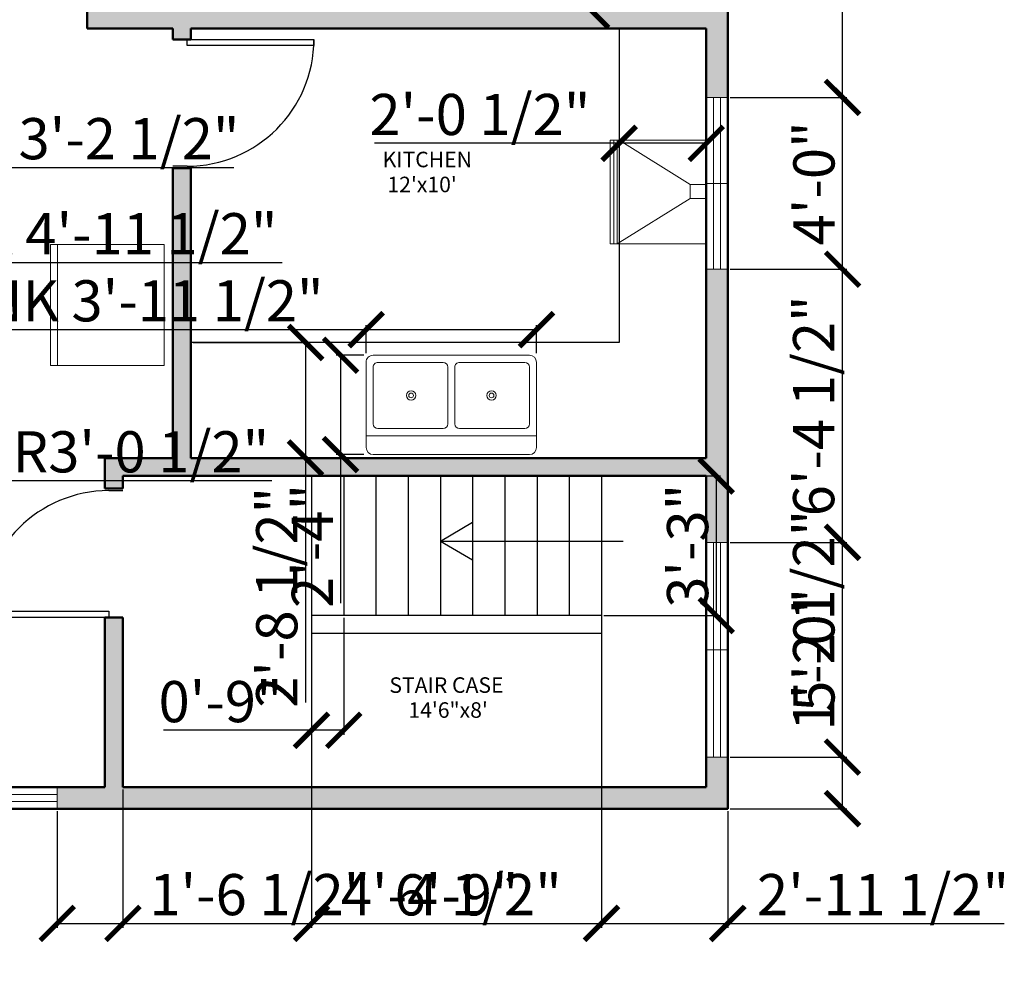
# Model space of a CAD drawing. Units: inches. Extents: x 3147 to 3847, y 1414 to 2207.
# Tile 4 of 7: x 3572 to 3847, y 1452 to 1716. Entities that reach past the tile are written whole.
import ezdxf

# ---------------------------------------------------------------- set-up
doc = ezdxf.new("R2010")
doc.units = ezdxf.units.IN
for name, color, linetype, lineweight in [('A-ANNO-DIMS', 2, 'Continuous', 18), ('A-AREA-IDEN', 7, 'Continuous', 18), ('A-DOOR', 3, 'Continuous', 25), ('A-EQPM', 9, 'Continuous', 18), ('A-FLOR-CASE', 32, 'Continuous', 25), ('A-FLOR-FIXT', 9, 'Continuous', 18), ('A-FLOR-STRS', 7, 'Continuous', 25), ('A-GLAZ', 4, 'Continuous', 18), ('A-WALL', 7, 'Continuous', 50)]:
    doc.layers.add(name, color=color, linetype=linetype, lineweight=lineweight)
doc.layers.add('A-WALL-PATT', color=18, linetype='Continuous', lineweight=13, true_color=0x000000)
doc.styles.get("Standard").update_dxf_attribs({"font": 'arial.ttf'})
doc.dimstyles.new('ISO-25', dxfattribs={"dimtxt": 11.5, "dimasz": 9.5, "dimexe": 1.25, "dimexo": 0.625, "dimtad": 1, "dimdec": 0, "dimlunit": 3, "dimtxsty": 'Standard', "dimblk": 'ARCHTICK', "dimcen": 2.5, "dimadec": 0, "dimazin": 0, "dimtfac": 1, "dimtdec": 0, "dimtmove": 0, "dimatfit": 3, "dimfxl": 1, "dimarcsym": 0})

# ---------------------------------------------------------------- blocks, each defined once
blk = doc.blocks.new('*U6')
for p, q in [((0, 0), (0, -100)), ((900, 0), (900, -100))]:
    blk.add_line(p, q)
blk.add_lwpolyline([(0, 0), (0, 900), (43.75, 900), (43.75, 0)], close=True)
blk.add_arc((0, 0), 900, 0, 90)
blk = doc.blocks.new('Sink-double - 36 in top')
for p, q in [((-18, -4), (18, -4)), ((-0.75, -18.5), (-0.75, -6.5)), ((0.75, -6.5), (0.75, -18.5))]:
    blk.add_line(p, q)
for points in [[(-16.5, 0), (16.5, 0)], [(-18, -19.5), (-18, -1.5)], [(18, -1.5), (18, -19.5)], [(-15.5, -5.5), (-1.75, -5.5)], [(1.75, -5.5), (15.5, -5.5)], [(-16.5, -18.5), (-16.5, -6.5)], [(16.5, -6.5), (16.5, -18.5)], [(-1.75, -19.5), (-15.5, -19.5)], [(15.5, -19.5), (1.75, -19.5)], [(16.5, -21), (-16.5, -21)]]:
    blk.add_lwpolyline(points)
for centre, radius in [((-8.5, -12.5), 1), ((-8.5, -12.5), 0.5), ((8.5, -12.5), 1), ((8.5, -12.5), 0.5)]:
    blk.add_circle(centre, radius)
for centre, radius, start, end in [((-16.5, -1.5), 1.5, 90, 180), ((16.5, -1.5), 1.5, 0, 90), ((-15.5, -6.5), 1, 90, 180), ((-1.75, -6.5), 1, 0, 90), ((1.75, -6.5), 1, 90, 180), ((15.5, -6.5), 1, 0, 90), ((-15.5, -18.5), 1, 180, 270), ((-1.75, -18.5), 1, 270, 0), ((1.75, -18.5), 1, 180, 270), ((15.5, -18.5), 1, 270, 0), ((-16.5, -19.5), 1.5, 180, 270), ((16.5, -19.5), 1.5, 270, 0)]:
    blk.add_arc(centre, radius, start, end)
blk = doc.blocks.new('WIN-48IN-DIVIDED')
for p, q in [((0, 6), (0, 0)), ((24, 6), (24, 0)), ((48, 6), (48, 0)), ((48, 4), (0, 4))]:
    blk.add_line(p, q)
blk.add_lwpolyline([(48, 2), (0, 2)])
blk = doc.blocks.new('_ArchTick')
at = {"color": 0, "linetype": 'ByBlock', "const_width": 0.15}
blk.add_lwpolyline([(-0.5, -0.5), (0.5, 0.5)], dxfattribs=at)
blk = doc.blocks.new('*D41')
at = {"layer": 'A-ANNO-DIMS', "color": 0, "lineweight": -2, "transparency": 16777216}
for p, q in [((3460.68, 1639.4), (3460.68, 1648.92)), ((3520.02, 1639.4), (3520.02, 1648.92)), ((3460.68, 1647.67), (3520.02, 1647.67)), ((3520.02, 1647.67), (3645.23, 1647.67))]:
    blk.add_line(p, q, dxfattribs=at)
at = {"layer": 'Defpoints', "color": 0, "transparency": 16777216}
for p in [(3520.02, 1647.67), (3460.68, 1638.77), (3520.02, 1638.77)]:
    blk.add_point(p, dxfattribs=at)
at = {"layer": 'A-ANNO-DIMS', "color": 0, "lineweight": -2, "transparency": 16777216, "xscale": 9.5, "yscale": 9.5, "zscale": 9.5, "rotation": 180}
blk.add_blockref('_ArchTick', (3460.68, 1647.67), dxfattribs=at)
at = {"layer": 'A-ANNO-DIMS', "color": 0, "lineweight": -2, "transparency": 16777216, "xscale": 9.5, "yscale": 9.5, "zscale": 9.5}
blk.add_blockref('_ArchTick', (3520.02, 1647.67), dxfattribs=at)
at = {"layer": 'A-ANNO-DIMS', "color": 0, "transparency": 16777216, "insert": (3587.38, 1654.25), "char_height": 11.5, "attachment_point": 5}
blk.add_mtext('SOFA 4\'-11 1/2"', dxfattribs=at)
blk = doc.blocks.new('*D45')
at = {"layer": 'A-ANNO-DIMS', "color": 0, "lineweight": -2, "transparency": 16777216}
for p, q in [((3668.72, 1628.92), (3479.75, 1628.92)), ((3668.72, 1622.4), (3668.72, 1630.17)), ((3716.33, 1628.92), (3668.72, 1628.92)), ((3716.33, 1622.4), (3716.33, 1630.17))]:
    blk.add_line(p, q, dxfattribs=at)
at = {"layer": 'Defpoints', "color": 0, "transparency": 16777216}
for p in [(3668.72, 1628.92), (3668.72, 1621.78), (3716.33, 1621.78)]:
    blk.add_point(p, dxfattribs=at)
at = {"layer": 'A-ANNO-DIMS', "color": 0, "lineweight": -2, "transparency": 16777216, "xscale": 9.5, "yscale": 9.5, "zscale": 9.5, "rotation": 180}
blk.add_blockref('_ArchTick', (3668.72, 1628.92), dxfattribs=at)
at = {"layer": 'A-ANNO-DIMS', "color": 0, "lineweight": -2, "transparency": 16777216, "xscale": 9.5, "yscale": 9.5, "zscale": 9.5}
blk.add_blockref('_ArchTick', (3716.33, 1628.92), dxfattribs=at)
at = {"layer": 'A-ANNO-DIMS', "color": 0, "transparency": 16777216, "insert": (3569.49, 1635.5), "char_height": 11.5, "attachment_point": 5}
blk.add_mtext('DOUBLE SINK 3\'-11 1/2"', dxfattribs=at)
blk = doc.blocks.new('*D46')
at = {"layer": 'A-ANNO-DIMS', "color": 0, "lineweight": -2, "transparency": 16777216}
for p, q in [((3668.1, 1621.78), (3660.33, 1621.78)), ((3661.58, 1621.78), (3661.58, 1594.01)), ((3668.1, 1594.01), (3660.33, 1594.01)), ((3661.58, 1594.01), (3661.58, 1552.49))]:
    blk.add_line(p, q, dxfattribs=at)
at = {"layer": 'Defpoints', "color": 0, "transparency": 16777216}
for p in [(3668.72, 1621.78), (3661.58, 1594.01), (3668.72, 1594.01)]:
    blk.add_point(p, dxfattribs=at)
at = {"layer": 'A-ANNO-DIMS', "color": 0, "lineweight": -2, "transparency": 16777216, "xscale": 9.5, "yscale": 9.5, "zscale": 9.5}
for p, rotation in [((3661.58, 1621.78), 90), ((3661.58, 1594.01), 270)]:
    blk.add_blockref('_ArchTick', p, dxfattribs=dict(at, rotation=rotation))
at = {"layer": 'A-ANNO-DIMS', "color": 0, "transparency": 16777216, "insert": (3655.18, 1568.5), "char_height": 11.5, "attachment_point": 5, "rotation": 90}
blk.add_mtext('2\'-4"', dxfattribs=at)
blk = doc.blocks.new('*D50')
at = {"layer": 'A-ANNO-DIMS', "color": 0, "lineweight": -2, "transparency": 16777216}
for p, q in [((3525.21, 1683.16), (3525.21, 1672.98)), ((3563.68, 1683.16), (3563.68, 1672.98)), ((3525.21, 1674.23), (3563.68, 1674.23)), ((3563.68, 1674.23), (3631.79, 1674.23))]:
    blk.add_line(p, q, dxfattribs=at)
at = {"layer": 'Defpoints', "color": 0, "transparency": 16777216}
for p in [(3525.21, 1683.78), (3563.68, 1683.78), (3563.68, 1674.23)]:
    blk.add_point(p, dxfattribs=at)
at = {"layer": 'A-ANNO-DIMS', "color": 0, "lineweight": -2, "transparency": 16777216, "xscale": 9.5, "yscale": 9.5, "zscale": 9.5, "rotation": 180}
blk.add_blockref('_ArchTick', (3525.21, 1674.23), dxfattribs=at)
at = {"layer": 'A-ANNO-DIMS', "color": 0, "lineweight": -2, "transparency": 16777216, "xscale": 9.5, "yscale": 9.5, "zscale": 9.5}
blk.add_blockref('_ArchTick', (3563.68, 1674.23), dxfattribs=at)
at = {"layer": 'A-ANNO-DIMS', "color": 0, "transparency": 16777216, "insert": (3602.48, 1680.81), "char_height": 11.5, "attachment_point": 5}
blk.add_mtext('3\'-2 1/2"', dxfattribs=at)
blk = doc.blocks.new('*D52')
at = {"layer": 'A-ANNO-DIMS', "color": 0, "lineweight": -2, "transparency": 16777216}
for p, q in [((3801.81, 1509.48), (3801.81, 1576.51)), ((3770.39, 1509.48), (3803.06, 1509.48)), ((3801.81, 1495.05), (3801.81, 1509.48)), ((3770.39, 1495.05), (3803.06, 1495.05))]:
    blk.add_line(p, q, dxfattribs=at)
at = {"layer": 'Defpoints', "color": 0, "transparency": 16777216}
for p in [(3769.76, 1509.48), (3801.81, 1509.48), (3769.76, 1495.05)]:
    blk.add_point(p, dxfattribs=at)
at = {"layer": 'A-ANNO-DIMS', "color": 0, "lineweight": -2, "transparency": 16777216, "xscale": 9.5, "yscale": 9.5, "zscale": 9.5}
for p, rotation in [((3801.81, 1509.48), 90), ((3801.81, 1495.05), 270)]:
    blk.add_blockref('_ArchTick', p, dxfattribs=dict(at, rotation=rotation))
at = {"layer": 'A-ANNO-DIMS', "color": 0, "transparency": 16777216, "insert": (3795.24, 1547.75), "char_height": 11.5, "attachment_point": 5, "rotation": 90}
blk.add_mtext('1\'-2 1/2"', dxfattribs=at)
blk = doc.blocks.new('*D53')
at = {"layer": 'A-ANNO-DIMS', "color": 0, "lineweight": -2, "transparency": 16777216}
for p, q in [((3770.39, 1569.48), (3803.06, 1569.48)), ((3801.81, 1509.48), (3801.81, 1569.48)), ((3770.39, 1509.48), (3803.06, 1509.48))]:
    blk.add_line(p, q, dxfattribs=at)
at = {"layer": 'Defpoints', "color": 0, "transparency": 16777216}
for p in [(3769.76, 1569.48), (3801.81, 1569.48), (3769.76, 1509.48)]:
    blk.add_point(p, dxfattribs=at)
at = {"layer": 'A-ANNO-DIMS', "color": 0, "lineweight": -2, "transparency": 16777216, "xscale": 9.5, "yscale": 9.5, "zscale": 9.5}
for p, rotation in [((3801.81, 1569.48), 90), ((3801.81, 1509.48), 270)]:
    blk.add_blockref('_ArchTick', p, dxfattribs=dict(at, rotation=rotation))
at = {"layer": 'A-ANNO-DIMS', "color": 0, "transparency": 16777216, "insert": (3795.32, 1539.48), "char_height": 11.5, "attachment_point": 5, "rotation": 90}
blk.add_mtext('5\'-0"', dxfattribs=at)
blk = doc.blocks.new('*D54')
at = {"layer": 'A-ANNO-DIMS', "color": 0, "lineweight": -2, "transparency": 16777216}
for p, q in [((3770.39, 1645.82), (3803.06, 1645.82)), ((3801.81, 1569.48), (3801.81, 1645.82)), ((3770.39, 1569.48), (3803.06, 1569.48))]:
    blk.add_line(p, q, dxfattribs=at)
at = {"layer": 'Defpoints', "color": 0, "transparency": 16777216}
for p in [(3769.76, 1645.82), (3801.81, 1645.82), (3769.76, 1569.48)]:
    blk.add_point(p, dxfattribs=at)
at = {"layer": 'A-ANNO-DIMS', "color": 0, "lineweight": -2, "transparency": 16777216, "xscale": 9.5, "yscale": 9.5, "zscale": 9.5}
for p, rotation in [((3801.81, 1645.82), 90), ((3801.81, 1569.48), 270)]:
    blk.add_blockref('_ArchTick', p, dxfattribs=dict(at, rotation=rotation))
at = {"layer": 'A-ANNO-DIMS', "color": 0, "transparency": 16777216, "insert": (3795.24, 1607.65), "char_height": 11.5, "attachment_point": 5, "rotation": 90}
blk.add_mtext('6\'-4 1/2"', dxfattribs=at)
blk = doc.blocks.new('*D55')
at = {"layer": 'A-ANNO-DIMS', "color": 0, "lineweight": -2, "transparency": 16777216}
for p, q in [((3770.39, 1693.82), (3803.06, 1693.82)), ((3801.81, 1645.82), (3801.81, 1693.82)), ((3770.39, 1645.82), (3803.06, 1645.82))]:
    blk.add_line(p, q, dxfattribs=at)
at = {"layer": 'Defpoints', "color": 0, "transparency": 16777216}
for p in [(3769.76, 1693.82), (3801.81, 1693.82), (3769.76, 1645.82)]:
    blk.add_point(p, dxfattribs=at)
at = {"layer": 'A-ANNO-DIMS', "color": 0, "lineweight": -2, "transparency": 16777216, "xscale": 9.5, "yscale": 9.5, "zscale": 9.5}
for p, rotation in [((3801.81, 1693.82), 90), ((3801.81, 1645.82), 270)]:
    blk.add_blockref('_ArchTick', p, dxfattribs=dict(at, rotation=rotation))
at = {"layer": 'A-ANNO-DIMS', "color": 0, "transparency": 16777216, "insert": (3795.32, 1669.82), "char_height": 11.5, "attachment_point": 5, "rotation": 90}
blk.add_mtext('4\'-0"', dxfattribs=at)
blk = doc.blocks.new('*D56')
at = {"layer": 'A-ANNO-DIMS', "color": 0, "lineweight": -2, "transparency": 16777216}
for p, q in [((3801.81, 1731.24), (3801.81, 1799.35)), ((3770.39, 1731.24), (3803.06, 1731.24)), ((3801.81, 1693.82), (3801.81, 1731.24)), ((3770.39, 1693.82), (3803.06, 1693.82))]:
    blk.add_line(p, q, dxfattribs=at)
at = {"layer": 'Defpoints', "color": 0, "transparency": 16777216}
for p in [(3769.76, 1731.24), (3801.81, 1731.24), (3769.76, 1693.82)]:
    blk.add_point(p, dxfattribs=at)
at = {"layer": 'A-ANNO-DIMS', "color": 0, "lineweight": -2, "transparency": 16777216, "xscale": 9.5, "yscale": 9.5, "zscale": 9.5}
for p, rotation in [((3801.81, 1731.24), 90), ((3801.81, 1693.82), 270)]:
    blk.add_blockref('_ArchTick', p, dxfattribs=dict(at, rotation=rotation))
at = {"layer": 'A-ANNO-DIMS', "color": 0, "transparency": 16777216, "insert": (3795.24, 1770.05), "char_height": 11.5, "attachment_point": 5, "rotation": 90}
blk.add_mtext('3\'-1 1/2"', dxfattribs=at)
blk = doc.blocks.new('*D71')
at = {"layer": 'A-ANNO-DIMS', "color": 0, "lineweight": -2, "transparency": 16777216}
for p, q in [((3600.76, 1500.42), (3600.76, 1461.75)), ((3582.41, 1494.42), (3582.41, 1461.75)), ((3582.41, 1463), (3600.76, 1463)), ((3600.76, 1463), (3667.8, 1463))]:
    blk.add_line(p, q, dxfattribs=at)
at = {"layer": 'Defpoints', "color": 0, "transparency": 16777216}
for p in [(3600.76, 1501.05), (3582.41, 1495.05), (3600.76, 1463)]:
    blk.add_point(p, dxfattribs=at)
at = {"layer": 'A-ANNO-DIMS', "color": 0, "lineweight": -2, "transparency": 16777216, "xscale": 9.5, "yscale": 9.5, "zscale": 9.5, "rotation": 180}
blk.add_blockref('_ArchTick', (3582.41, 1463), dxfattribs=at)
at = {"layer": 'A-ANNO-DIMS', "color": 0, "lineweight": -2, "transparency": 16777216, "xscale": 9.5, "yscale": 9.5, "zscale": 9.5}
blk.add_blockref('_ArchTick', (3600.76, 1463), dxfattribs=at)
at = {"layer": 'A-ANNO-DIMS', "color": 0, "transparency": 16777216, "insert": (3639.03, 1469.57), "char_height": 11.5, "attachment_point": 5}
blk.add_mtext('1\'-6 1/2"', dxfattribs=at)
blk = doc.blocks.new('*D72')
at = {"layer": 'A-ANNO-DIMS', "color": 0, "lineweight": -2, "transparency": 16777216}
for p, q in [((3653.47, 1548.42), (3653.47, 1461.75)), ((3600.76, 1500.42), (3600.76, 1461.75)), ((3600.76, 1463), (3653.47, 1463)), ((3653.47, 1463), (3722.05, 1463))]:
    blk.add_line(p, q, dxfattribs=at)
at = {"layer": 'Defpoints', "color": 0, "transparency": 16777216}
for p in [(3653.47, 1549.05), (3600.76, 1501.05), (3653.47, 1463)]:
    blk.add_point(p, dxfattribs=at)
at = {"layer": 'A-ANNO-DIMS', "color": 0, "lineweight": -2, "transparency": 16777216, "xscale": 9.5, "yscale": 9.5, "zscale": 9.5, "rotation": 180}
blk.add_blockref('_ArchTick', (3600.76, 1463), dxfattribs=at)
at = {"layer": 'A-ANNO-DIMS', "color": 0, "lineweight": -2, "transparency": 16777216, "xscale": 9.5, "yscale": 9.5, "zscale": 9.5}
blk.add_blockref('_ArchTick', (3653.47, 1463), dxfattribs=at)
at = {"layer": 'A-ANNO-DIMS', "color": 0, "transparency": 16777216, "insert": (3692.51, 1469.57), "char_height": 11.5, "attachment_point": 5}
blk.add_mtext('4\'-4 1/2"', dxfattribs=at)
blk = doc.blocks.new('*D73')
at = {"layer": 'A-ANNO-DIMS', "color": 0, "lineweight": -2, "transparency": 16777216}
for p, q in [((3653.47, 1548.42), (3653.47, 1461.75)), ((3734.47, 1548.42), (3734.47, 1461.75)), ((3653.47, 1463), (3734.47, 1463))]:
    blk.add_line(p, q, dxfattribs=at)
at = {"layer": 'Defpoints', "color": 0, "transparency": 16777216}
for p in [(3653.47, 1549.05), (3734.47, 1549.05), (3734.47, 1463)]:
    blk.add_point(p, dxfattribs=at)
at = {"layer": 'A-ANNO-DIMS', "color": 0, "lineweight": -2, "transparency": 16777216, "xscale": 9.5, "yscale": 9.5, "zscale": 9.5, "rotation": 180}
blk.add_blockref('_ArchTick', (3653.47, 1463), dxfattribs=at)
at = {"layer": 'A-ANNO-DIMS', "color": 0, "lineweight": -2, "transparency": 16777216, "xscale": 9.5, "yscale": 9.5, "zscale": 9.5}
blk.add_blockref('_ArchTick', (3734.47, 1463), dxfattribs=at)
at = {"layer": 'A-ANNO-DIMS', "color": 0, "transparency": 16777216, "insert": (3693.97, 1469.5), "char_height": 11.5, "attachment_point": 5}
blk.add_mtext('6\'-9"', dxfattribs=at)
blk = doc.blocks.new('*D74')
at = {"layer": 'A-ANNO-DIMS', "color": 0, "lineweight": -2, "transparency": 16777216}
for p, q in [((3734.47, 1548.42), (3734.47, 1461.75)), ((3769.76, 1494.42), (3769.76, 1461.75)), ((3734.47, 1463), (3769.76, 1463)), ((3769.76, 1463), (3847.01, 1463))]:
    blk.add_line(p, q, dxfattribs=at)
at = {"layer": 'Defpoints', "color": 0, "transparency": 16777216}
for p in [(3734.47, 1549.05), (3769.76, 1495.05), (3769.76, 1463)]:
    blk.add_point(p, dxfattribs=at)
at = {"layer": 'A-ANNO-DIMS', "color": 0, "lineweight": -2, "transparency": 16777216, "xscale": 9.5, "yscale": 9.5, "zscale": 9.5, "rotation": 180}
blk.add_blockref('_ArchTick', (3734.47, 1463), dxfattribs=at)
at = {"layer": 'A-ANNO-DIMS', "color": 0, "lineweight": -2, "transparency": 16777216, "xscale": 9.5, "yscale": 9.5, "zscale": 9.5}
blk.add_blockref('_ArchTick', (3769.76, 1463), dxfattribs=at)
at = {"layer": 'A-ANNO-DIMS', "color": 0, "transparency": 16777216, "insert": (3813.14, 1469.57), "char_height": 11.5, "attachment_point": 5}
blk.add_mtext('2\'-11 1/2"', dxfattribs=at)
blk = doc.blocks.new('*D88')
at = {"layer": 'A-ANNO-DIMS', "color": 0, "lineweight": -2, "transparency": 16777216}
for p, q in [((3763.14, 1849.05), (3730.46, 1849.05)), ((3731.71, 1718.05), (3731.71, 1849.05)), ((3763.14, 1718.05), (3730.46, 1718.05))]:
    blk.add_line(p, q, dxfattribs=at)
at = {"layer": 'Defpoints', "color": 0, "transparency": 16777216}
for p in [(3731.71, 1849.05), (3763.76, 1849.05), (3763.76, 1718.05)]:
    blk.add_point(p, dxfattribs=at)
at = {"layer": 'A-ANNO-DIMS', "color": 0, "lineweight": -2, "transparency": 16777216, "xscale": 9.5, "yscale": 9.5, "zscale": 9.5}
for p, rotation in [((3731.71, 1849.05), 90), ((3731.71, 1718.05), 270)]:
    blk.add_blockref('_ArchTick', p, dxfattribs=dict(at, rotation=rotation))
at = {"layer": 'A-ANNO-DIMS', "color": 0, "transparency": 16777216, "insert": (3725.22, 1783.55), "char_height": 11.5, "attachment_point": 5, "rotation": 90}
blk.add_mtext('10\'-11"', dxfattribs=at)
blk = doc.blocks.new('*D90')
at = {"layer": 'A-ANNO-DIMS', "color": 0, "lineweight": -2, "transparency": 16777216}
for p, q in [((3735.1, 1588.05), (3767.77, 1588.05)), ((3766.52, 1588.05), (3766.52, 1549.05)), ((3735.1, 1549.05), (3767.77, 1549.05))]:
    blk.add_line(p, q, dxfattribs=at)
at = {"layer": 'Defpoints', "color": 0, "transparency": 16777216}
for p in [(3734.47, 1588.05), (3734.47, 1549.05), (3766.52, 1549.05)]:
    blk.add_point(p, dxfattribs=at)
at = {"layer": 'A-ANNO-DIMS', "color": 0, "lineweight": -2, "transparency": 16777216, "xscale": 9.5, "yscale": 9.5, "zscale": 9.5}
for p, rotation in [((3766.52, 1588.05), 90), ((3766.52, 1549.05), 270)]:
    blk.add_blockref('_ArchTick', p, dxfattribs=dict(at, rotation=rotation))
at = {"layer": 'A-ANNO-DIMS', "color": 0, "transparency": 16777216, "insert": (3760.02, 1568.55), "char_height": 11.5, "attachment_point": 5, "rotation": 90}
blk.add_mtext('3\'-3"', dxfattribs=at)
blk = doc.blocks.new('*D91')
at = {"layer": 'A-ANNO-DIMS', "color": 0, "lineweight": -2, "transparency": 16777216}
for p, q in [((3653.47, 1548.42), (3653.47, 1515.75)), ((3662.47, 1548.42), (3662.47, 1515.75)), ((3653.47, 1517), (3612.15, 1517)), ((3662.47, 1517), (3653.47, 1517))]:
    blk.add_line(p, q, dxfattribs=at)
at = {"layer": 'Defpoints', "color": 0, "transparency": 16777216}
for p in [(3653.47, 1549.05), (3662.47, 1549.05), (3653.47, 1517)]:
    blk.add_point(p, dxfattribs=at)
at = {"layer": 'A-ANNO-DIMS', "color": 0, "lineweight": -2, "transparency": 16777216, "xscale": 9.5, "yscale": 9.5, "zscale": 9.5, "rotation": 180}
blk.add_blockref('_ArchTick', (3653.47, 1517), dxfattribs=at)
at = {"layer": 'A-ANNO-DIMS', "color": 0, "lineweight": -2, "transparency": 16777216, "xscale": 9.5, "yscale": 9.5, "zscale": 9.5}
blk.add_blockref('_ArchTick', (3662.47, 1517), dxfattribs=at)
at = {"layer": 'A-ANNO-DIMS', "color": 0, "transparency": 16777216, "insert": (3628.06, 1523.5), "char_height": 11.5, "attachment_point": 5}
blk.add_mtext('0\'-9"', dxfattribs=at)
blk = doc.blocks.new('*D92')
at = {"layer": 'A-ANNO-DIMS', "color": 0, "lineweight": -2, "transparency": 16777216}
for p, q in [((3620.39, 1625.36), (3653.06, 1625.36)), ((3651.81, 1625.36), (3651.81, 1593.05)), ((3620.39, 1593.05), (3653.06, 1593.05)), ((3651.81, 1593.05), (3651.81, 1524.74))]:
    blk.add_line(p, q, dxfattribs=at)
at = {"layer": 'Defpoints', "color": 0, "transparency": 16777216}
for p in [(3619.76, 1625.36), (3619.76, 1593.05), (3651.81, 1593.05)]:
    blk.add_point(p, dxfattribs=at)
at = {"layer": 'A-ANNO-DIMS', "color": 0, "lineweight": -2, "transparency": 16777216, "xscale": 9.5, "yscale": 9.5, "zscale": 9.5}
for p, rotation in [((3651.81, 1625.36), 90), ((3651.81, 1593.05), 270)]:
    blk.add_blockref('_ArchTick', p, dxfattribs=dict(at, rotation=rotation))
at = {"layer": 'A-ANNO-DIMS', "color": 0, "transparency": 16777216, "insert": (3645.24, 1554.14), "char_height": 11.5, "attachment_point": 5, "rotation": 90}
blk.add_mtext('2\'-8 1/2"', dxfattribs=at)
blk = doc.blocks.new('*D93')
at = {"layer": 'A-ANNO-DIMS', "color": 0, "lineweight": -2, "transparency": 16777216}
for p, q in [((3739.42, 1712.42), (3739.42, 1679.75)), ((3763.76, 1712.42), (3763.76, 1679.75)), ((3739.42, 1681), (3671.1, 1681)), ((3763.76, 1681), (3739.42, 1681))]:
    blk.add_line(p, q, dxfattribs=at)
at = {"layer": 'Defpoints', "color": 0, "transparency": 16777216}
for p in [(3739.42, 1713.05), (3763.76, 1713.05), (3739.42, 1681)]:
    blk.add_point(p, dxfattribs=at)
at = {"layer": 'A-ANNO-DIMS', "color": 0, "lineweight": -2, "transparency": 16777216, "xscale": 9.5, "yscale": 9.5, "zscale": 9.5, "rotation": 180}
blk.add_blockref('_ArchTick', (3739.42, 1681), dxfattribs=at)
at = {"layer": 'A-ANNO-DIMS', "color": 0, "lineweight": -2, "transparency": 16777216, "xscale": 9.5, "yscale": 9.5, "zscale": 9.5}
blk.add_blockref('_ArchTick', (3763.76, 1681), dxfattribs=at)
at = {"layer": 'A-ANNO-DIMS', "color": 0, "transparency": 16777216, "insert": (3700.51, 1687.57), "char_height": 11.5, "attachment_point": 5}
blk.add_mtext('2\'-0 1/2"', dxfattribs=at)
blk = doc.blocks.new('*D98')
at = {"layer": 'A-ANNO-DIMS', "color": 0, "lineweight": -2, "transparency": 16777216}
for p in [(3492.69, 1586.73), (3642.35, 1586.73)]:
    blk.add_line(p, (3529.03, 1586.73), dxfattribs=at)
at = {"layer": 'Defpoints', "color": 0, "transparency": 16777216}
for p in [(3492.69, 1586.73), (3529.03, 1586.73)]:
    blk.add_point(p, dxfattribs=at)
at = {"layer": 'A-ANNO-DIMS', "color": 0, "lineweight": -2, "transparency": 16777216, "xscale": 9.5, "yscale": 9.5, "zscale": 9.5, "rotation": 180.0000425795118}
blk.add_blockref('_ArchTick', (3529.03, 1586.73), dxfattribs=at)
at = {"layer": 'A-ANNO-DIMS', "color": 0, "transparency": 16777216, "insert": (3595.19, 1593.3), "char_height": 11.5, "attachment_point": 5, "rotation": 0}
blk.add_mtext('3X R3\'-0 1/2"', dxfattribs=at)

msp = doc.modelspace()

# ---------------------------------------------------------------- hatches: boundary and pattern name
at = {"layer": 'A-WALL-PATT'}
h = msp.add_hatch(color=256, dxfattribs=at)
h.dxf.hatch_style = 1
h.paths.add_polyline_path([(3616.76, 2093.05), (3594.02, 2093.05), (3594.02, 2087.05), (3611.76, 2087.05), (3611.76, 1993.05), (3616.76, 1993.05), (3628.76, 1993.05), (3628.76, 1996.99), (3628.76, 1998.05), (3616.76, 1998.05), (3616.76, 2087.05)])
h.paths.add_polyline_path([(3576.44, 2093.05), (3527.03, 2093.05), (3527.03, 2087.05), (3546.76, 2087.05), (3546.76, 1962.05), (3551.76, 1962.05), (3590.76, 1962.05), (3590.76, 1921.05), (3585.76, 1921.05), (3585.76, 1916.05), (3590.76, 1916.05), (3590.76, 1895.05), (3595.76, 1895.05), (3595.76, 1962.05), (3611.76, 1962.05), (3616.76, 1962.05), (3616.76, 1969.05), (3611.76, 1969.05), (3611.76, 1967.05), (3551.76, 1967.05), (3551.76, 2087.05), (3576.44, 2087.05)])
h.paths.add_polyline_path([(3455.03, 2093.05), (3408.76, 2093.05), (3408.76, 2087.05), (3408.76, 2046.06), (3413.76, 2046.06), (3413.76, 2087.05), (3455.03, 2087.05)])
h.paths.add_polyline_path([(3355.76, 2008.05), (3408.76, 2008.05), (3408.76, 2004.83), (3413.76, 2004.83), (3413.76, 2008.05), (3413.76, 2013.05), (3413.76, 2016.06), (3408.76, 2016.06), (3408.76, 2013.05), (3355.76, 2013.05), (3349.76, 2013.05), (3349.76, 1973.71), (3355.76, 1973.71)])
h.paths.add_polyline_path([(3413.76, 1974.83), (3408.76, 1974.83), (3408.76, 1943.05), (3355.76, 1943.05), (3355.76, 1949.71), (3349.76, 1949.71), (3349.76, 1897.34), (3355.76, 1897.34), (3355.76, 1938.05), (3408.76, 1938.05), (3408.76, 1934.63), (3413.76, 1934.63), (3413.76, 1938.05), (3505.76, 1938.05), (3505.76, 1916.05), (3533.76, 1916.05), (3533.76, 1904.63), (3533.76, 1831.83), (3538.76, 1831.83), (3538.76, 1904.63), (3538.76, 1916.05), (3546.76, 1916.05), (3549.76, 1916.05), (3549.76, 1921.05), (3546.76, 1921.05), (3510.76, 1921.05), (3510.76, 1938.05), (3510.76, 1943.05), (3413.76, 1943.05)])
h.paths.add_polyline_path([(3413.76, 1904.63), (3408.76, 1904.63), (3408.76, 1870.05), (3355.76, 1870.05), (3355.76, 1873.34), (3349.76, 1873.34), (3349.76, 1865.05), (3355.76, 1865.05), (3408.76, 1865.05), (3408.76, 1863.11), (3409.83, 1863.11), (3413.76, 1863.11)], flags=17)
h.paths.add_polyline_path([(3538.76, 1795.83), (3533.76, 1795.83), (3533.76, 1794.05), (3413.76, 1794.05), (3413.76, 1833.11), (3408.76, 1833.11), (3408.76, 1794.05), (3355.76, 1794.05), (3349.76, 1794.05), (3349.76, 1776.88), (3355.76, 1776.88), (3355.76, 1789.05), (3413.76, 1789.05), (3475.76, 1789.05), (3475.76, 1731.91), (3480.76, 1731.91), (3480.76, 1789.05), (3538.76, 1789.05)])
h.paths.add_polyline_path([(3432.14, 1733.05), (3413.76, 1733.05), (3355.76, 1733.05), (3355.76, 1740.88), (3349.76, 1740.88), (3349.76, 1720.47), (3355.76, 1720.47), (3355.76, 1729.05), (3413.76, 1729.05), (3432.14, 1729.05)])
h.paths.add_polyline_path([(3480.76, 1695.91), (3476.83, 1695.91), (3475.76, 1695.91), (3475.76, 1693.05), (3413.76, 1693.05), (3355.76, 1693.05), (3355.76, 1696.47), (3349.76, 1696.47), (3349.76, 1671.27), (3355.76, 1671.27), (3355.76, 1688.05), (3413.76, 1688.05), (3415.76, 1688.05), (3415.76, 1673.71), (3420.76, 1673.71), (3420.76, 1688.05), (3480.76, 1688.05)])
h.paths.add_polyline_path([(3420.76, 1643.71), (3415.76, 1643.71), (3415.76, 1642.05), (3413.76, 1642.05), (3355.76, 1642.05), (3355.76, 1647.27), (3349.76, 1647.27), (3349.76, 1598.35), (3355.76, 1598.35), (3355.76, 1637.05), (3401.76, 1637.05), (3401.76, 1634.26), (3406.76, 1634.26), (3406.76, 1637.05), (3413.76, 1637.05), (3420.76, 1637.05)])
h.paths.add_polyline_path([(3406.76, 1604.26), (3401.76, 1604.26), (3401.76, 1572.05), (3355.76, 1572.05), (3355.76, 1574.35), (3349.76, 1574.35), (3349.76, 1553.05), (3349.76, 1495.05), (3371.89, 1495.05), (3371.89, 1501.05), (3355.76, 1501.05), (3355.76, 1559.05), (3355.76, 1567.05), (3406.76, 1567.05), (3406.76, 1572.05)])
h.paths.add_polyline_path([(3534.41, 1501.05), (3419.89, 1501.05), (3419.89, 1495.05), (3534.41, 1495.05)])
h.paths.add_polyline_path([(3769.76, 1509.48), (3763.76, 1509.48), (3763.76, 1501.05), (3600.76, 1501.05), (3600.76, 1548.51), (3595.76, 1548.51), (3595.76, 1501.05), (3582.41, 1501.05), (3582.41, 1495.05), (3769.76, 1495.05)])
h.paths.add_polyline_path([(3769.76, 1645.82), (3763.76, 1645.82), (3763.76, 1593.05), (3664.76, 1593.05), (3619.76, 1593.05), (3619.76, 1674.05), (3614.76, 1674.05), (3614.76, 1593.05), (3595.76, 1593.05), (3595.76, 1584.51), (3600.76, 1584.51), (3600.76, 1588.05), (3619.76, 1588.05), (3664.76, 1588.05), (3763.76, 1588.05), (3763.76, 1569.48), (3769.76, 1569.48)])
h.paths.add_polyline_path([(3769.76, 1731.24), (3763.76, 1731.24), (3763.76, 1718.05), (3664.76, 1718.05), (3595.76, 1718.05), (3595.76, 1723.05), (3590.76, 1723.05), (3590.76, 1713.05), (3595.76, 1713.05), (3614.76, 1713.05), (3614.76, 1710.05), (3619.76, 1710.05), (3619.76, 1713.05), (3664.76, 1713.05), (3763.76, 1713.05), (3763.76, 1693.82), (3769.76, 1693.82)])
h.paths.add_polyline_path([(3769.76, 1872.64), (3763.76, 1872.64), (3763.76, 1854.05), (3664.76, 1854.05), (3595.76, 1854.05), (3595.76, 1859.05), (3590.76, 1859.05), (3590.76, 1759.05), (3595.76, 1759.05), (3595.76, 1849.05), (3664.76, 1849.05), (3763.76, 1849.05), (3763.76, 1815.24), (3769.76, 1815.24)])
h.paths.add_polyline_path([(3769.76, 1998.05), (3763.76, 1998.05), (3763.76, 1968.64), (3769.76, 1968.64)])
h.paths.add_polyline_path([(3763.76, 1998.05), (3664.76, 1998.05), (3664.76, 1993.05), (3763.76, 1993.05)])

# ---------------------------------------------------------------- linework, layer by layer
at = {"layer": 'A-EQPM'}
for p, q in [((3736.9, 1652.92), (3736.9, 1681.84)), ((3736.9, 1681.84), (3738.9, 1681.84)), ((3737.9, 1652.92), (3737.9, 1681.84)), ((3738.9, 1681.84), (3763.76, 1681.84)), ((3738.9, 1652.92), (3738.9, 1681.84)), ((3739.42, 1681.84), (3759.29, 1669.49)), ((3763.76, 1681.84), (3763.76, 1652.92)), ((3759.29, 1665.54), (3738.9, 1652.92)), ((3580.52, 1652.72), (3612.29, 1652.72)), ((3580.52, 1618.87), (3580.52, 1652.72)), ((3582.52, 1618.87), (3582.52, 1652.72)), ((3612.29, 1652.72), (3612.29, 1618.87)), ((3736.9, 1652.92), (3738.9, 1652.92)), ((3763.76, 1652.92), (3738.9, 1652.92)), ((3612.29, 1618.87), (3580.52, 1618.87))]:
    msp.add_line(p, q, dxfattribs=at)
msp.add_lwpolyline([(3759.29, 1669.49), (3763.76, 1669.49), (3763.76, 1665.54), (3759.29, 1665.54)], close=True, dxfattribs=at)
at = {"layer": 'A-FLOR-CASE'}
for p, q in [((3739.42, 1713.05), (3739.42, 1625.36)), ((3739.42, 1625.36), (3619.76, 1625.36))]:
    msp.add_line(p, q, dxfattribs=at)
at = {"layer": 'A-FLOR-STRS'}
for p, q in [((3653.47, 1588.05), (3653.47, 1501.05)), ((3662.47, 1588.05), (3662.47, 1549.05)), ((3671.47, 1588.05), (3671.47, 1549.05)), ((3680.47, 1588.05), (3680.47, 1549.05)), ((3689.47, 1588.05), (3689.47, 1549.05)), ((3698.47, 1588.05), (3698.47, 1549.05)), ((3707.47, 1588.05), (3707.47, 1549.05)), ((3716.47, 1588.05), (3716.47, 1549.05)), ((3725.47, 1588.05), (3725.47, 1549.05)), ((3734.47, 1588.05), (3734.47, 1501.05)), ((3689.47, 1569.85), (3698.47, 1575.11)), ((3689.47, 1569.85), (3698.47, 1564.59)), ((3689.47, 1569.85), (3740.56, 1569.85))]:
    msp.add_line(p, q, dxfattribs=at)
for points in [[(3734.47, 1549.05), (3664.76, 1549.05), (3653.47, 1549.05)], [(3734.47, 1544.05), (3664.76, 1544.05), (3653.47, 1544.05)]]:
    msp.add_lwpolyline(points, dxfattribs=at)
at = {"layer": 'A-GLAZ'}
for p, q in [((3763.76, 1693.82), (3769.76, 1693.82)), ((3765.76, 1693.82), (3765.76, 1645.82)), ((3767.76, 1693.82), (3767.76, 1645.82)), ((3763.76, 1669.82), (3769.76, 1669.82)), ((3763.76, 1645.82), (3769.76, 1645.82)), ((3763.76, 1569.48), (3769.76, 1569.48)), ((3765.76, 1569.48), (3765.76, 1509.48)), ((3767.76, 1569.48), (3767.76, 1553.05)), ((3763.76, 1539.48), (3769.76, 1539.48)), ((3763.76, 1509.48), (3769.76, 1509.48))]:
    msp.add_line(p, q, dxfattribs=at)
msp.add_lwpolyline([(3767.76, 1553.05), (3767.76, 1509.48)], dxfattribs=at)
at = {"layer": 'A-WALL'}
for p, q in [((3769.76, 2093.05), (3769.76, 1553.05)), ((3590.76, 1723.05), (3590.76, 1713.05)), ((3595.76, 1713.05), (3590.76, 1713.05)), ((3614.76, 1713.05), (3614.76, 1710.05)), ((3619.76, 1713.05), (3619.76, 1710.05)), ((3763.76, 1713.05), (3763.76, 1593.05)), ((3614.76, 1674.05), (3614.76, 1593.05)), ((3619.76, 1674.05), (3619.76, 1593.05)), ((3614.76, 1593.05), (3595.76, 1593.05)), ((3595.76, 1593.05), (3595.76, 1584.51)), ((3619.76, 1588.05), (3600.76, 1588.05)), ((3600.76, 1588.05), (3600.76, 1584.51)), ((3763.76, 1588.05), (3763.76, 1501.05)), ((3595.76, 1584.51), (3600.76, 1584.51)), ((3595.76, 1548.51), (3595.76, 1501.05)), ((3595.76, 1548.51), (3600.76, 1548.51)), ((3600.76, 1548.51), (3600.76, 1501.05)), ((3595.76, 1501.05), (3355.76, 1501.05)), ((3763.76, 1501.05), (3600.76, 1501.05))]:
    msp.add_line(p, q, dxfattribs=at)
for points in [[(3614.76, 1713.05), (3595.76, 1713.05)], [(3763.76, 1713.05), (3664.76, 1713.05), (3619.76, 1713.05)], [(3619.76, 1710.05), (3614.76, 1710.05)], [(3619.76, 1674.05), (3614.76, 1674.05)], [(3763.76, 1593.05), (3664.76, 1593.05), (3619.76, 1593.05)], [(3763.76, 1588.05), (3664.76, 1588.05), (3614.76, 1588.05)], [(3769.76, 1553.05), (3769.76, 1495.05), (3349.76, 1495.05), (3349.76, 1553.05)]]:
    msp.add_lwpolyline(points, dxfattribs=at)

# ---------------------------------------------------------------- block references
at = {"layer": 'A-DOOR', "xscale": 0.0393700787401575, "yscale": 0.0393700787401575, "zscale": 0.0393700787401575}
for p, rotation in [((3618.7, 1710.05), 270), ((3596.83, 1548.51), 89.99999999999999)]:
    msp.add_blockref('*U6', p, dxfattribs=dict(at, rotation=rotation))
at = {"layer": 'A-FLOR-FIXT', "xscale": 1.322443932435744, "yscale": 1.322443932435744, "zscale": 1.322443932435744, "rotation": 180}
msp.add_blockref('Sink-double - 36 in top', (3692.52, 1594.01), dxfattribs=at)
at = {"layer": 'A-GLAZ'}
msp.add_blockref('WIN-48IN-DIVIDED', (3534.41, 1495.05), dxfattribs=at)

# ---------------------------------------------------------------- texts
at = {"layer": 'A-AREA-IDEN'}
for s, height, p in [('KITCHEN', 4.34, (3673.33, 1674.3)), (" 12'x10'", 4.34, (3673.34, 1667.33)), ('STAIR CASE', 4.34, (3675.22, 1527.43)), ('    14\'6"x8\'', 4.3404, (3675.22, 1520.46))]:
    msp.add_text(s, height=height, rotation=0.0333, dxfattribs=at).set_placement(p)

# ---------------------------------------------------------------- dimensions: what is measured, and where the dimension line sits
at = {"layer": 'A-ANNO-DIMS'}
for base, p1, p2, angle, picture, middle in [((3731.71, 1849.05), (3763.76, 1718.05), (3763.76, 1849.05), 90, '*D88', (3725.22, 1783.55)), ((3801.81, 1731.24), (3769.76, 1693.82), (3769.76, 1731.24), 90, '*D56', (3795.24, 1770.05)), ((3739.42, 1681), (3763.76, 1713.05), (3739.42, 1713.05), 180, '*D93', (3700.51, 1687.57)), ((3801.81, 1693.82), (3769.76, 1645.82), (3769.76, 1693.82), 90, '*D55', (3795.32, 1669.82)), ((3801.81, 1645.82), (3769.76, 1569.48), (3769.76, 1645.82), 90, '*D54', (3795.24, 1607.65)), ((3651.81, 1593.05), (3619.76, 1625.36), (3619.76, 1593.05), 270, '*D92', (3645.24, 1554.14)), ((3661.58, 1594.01), (3668.72, 1621.78), (3668.72, 1594.01), 270, '*D46', (3655.18, 1568.5)), ((3766.52, 1549.05), (3734.47, 1588.05), (3734.47, 1549.05), 270, '*D90', (3760.02, 1568.55)), ((3801.81, 1509.48), (3769.76, 1495.05), (3769.76, 1509.48), 90, '*D52', (3795.24, 1547.75)), ((3801.81, 1569.48), (3769.76, 1509.48), (3769.76, 1569.48), 90, '*D53', (3795.32, 1539.48)), ((3653.47, 1517), (3662.47, 1549.05), (3653.47, 1549.05), 180, '*D91', (3628.06, 1523.5))]:
    dim = msp.add_linear_dim(base=base, p1=p1, p2=p2, angle=angle, dimstyle='ISO-25', override={"dimdec": 1, "dimlfac": 1, "dimrnd": 0, "dimzin": 1, "dimdsep": 46, "dimlunit": 4, "dimfrac": 2}, dxfattribs=at)
    dim.commit()
    dim.dimension.update_dxf_attribs({"geometry": picture, "text_midpoint": middle})
for base, p1, p2, picture, middle in [((3563.68, 1674.23), (3525.21, 1683.78), (3563.68, 1683.78), '*D50', (3602.48, 1680.81)), ((3653.47, 1463), (3600.76, 1501.05), (3653.47, 1549.05), '*D72', (3692.51, 1469.57)), ((3734.47, 1463), (3653.47, 1549.05), (3734.47, 1549.05), '*D73', (3693.97, 1469.5)), ((3769.76, 1463), (3734.47, 1549.05), (3769.76, 1495.05), '*D74', (3813.14, 1469.57)), ((3600.7645, 1462.9992), (3582.4102, 1495.0492), (3600.7645, 1501.0492), '*D71', (3639.0316, 1469.5703))]:
    dim = msp.add_linear_dim(base=base, p1=p1, p2=p2, dimstyle='ISO-25', override={"dimdec": 1, "dimlfac": 1, "dimrnd": 0, "dimzin": 1, "dimdsep": 46, "dimlunit": 4, "dimfrac": 2}, dxfattribs=at)
    dim.commit()
    dim.dimension.update_dxf_attribs({"geometry": picture, "text_midpoint": middle})
dim = msp.add_linear_dim(base=(3520.02, 1647.67), p1=(3460.68, 1638.77), p2=(3520.02, 1638.77), text='SOFA <>', dimstyle='ISO-25', override={"dimdec": 1, "dimlfac": 1, "dimrnd": 0, "dimzin": 1, "dimdsep": 46, "dimlunit": 4, "dimfrac": 2}, dxfattribs=at)
dim.commit()
dim.dimension.update_dxf_attribs({"geometry": '*D41', "text_midpoint": (3587.38, 1654.25)})
dim = msp.add_linear_dim(base=(3668.72, 1628.92), p1=(3716.33, 1621.78), p2=(3668.72, 1621.78), angle=180, text='DOUBLE SINK <>', dimstyle='ISO-25', override={"dimdec": 1, "dimlfac": 1, "dimrnd": 0, "dimzin": 1, "dimdsep": 46, "dimlunit": 4, "dimfrac": 2}, dxfattribs=at)
dim.commit()
dim.dimension.update_dxf_attribs({"geometry": '*D45', "text_midpoint": (3569.49, 1635.5)})
dim = msp.add_radius_dim(center=(3492.69, 1586.73), mpoint=(3529.03, 1586.73), text='3X <>', dimstyle='ISO-25', override={"dimdec": 1, "dimlfac": 1, "dimrnd": 0, "dimzin": 1, "dimdsep": 46, "dimlunit": 4, "dimfrac": 2}, dxfattribs=at)
dim.commit()
dim.dimension.update_dxf_attribs({"geometry": '*D98', "text_midpoint": (3595.19, 1593.3)})

doc.saveas('drawing.dxf')
